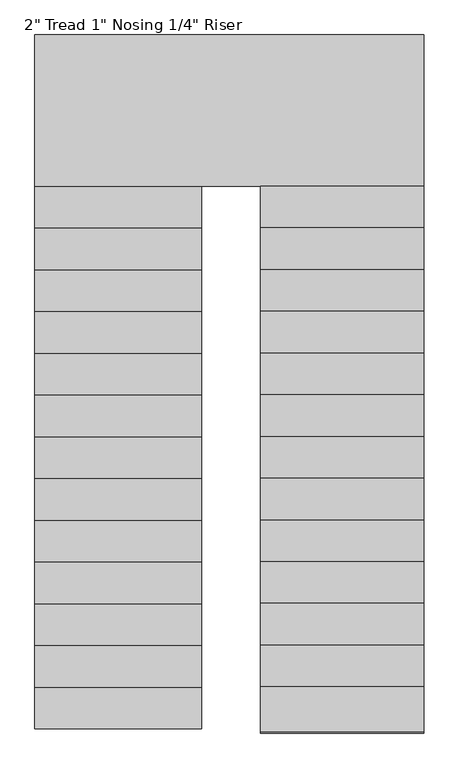
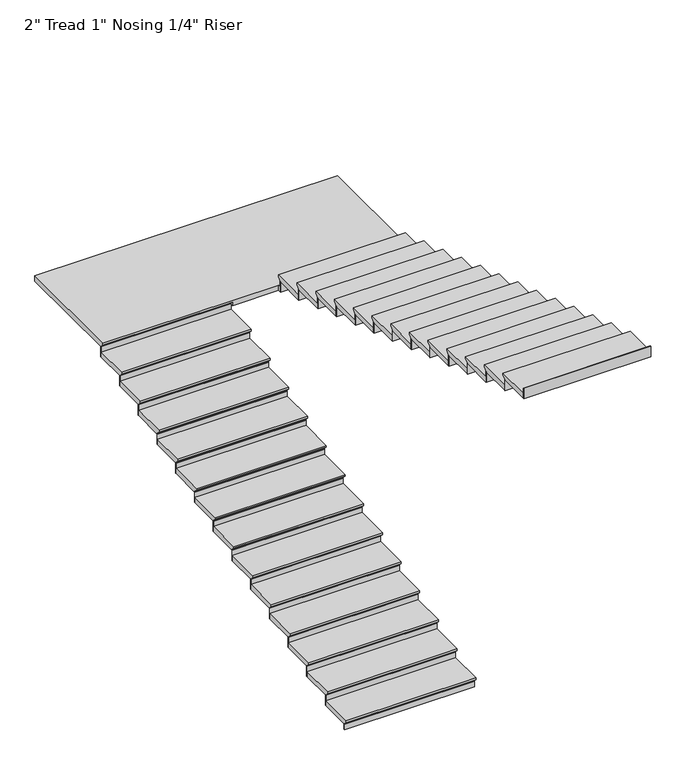
"""IFC4 building model written with IfcOpenShell, lengths in millimetres: stair flight geometry."""

from ifc_helpers import new_model, si_unit, origin, place, context, project, spatial, faceted_brep, source, transform, mapped, element, save


def stair_flight_1eae5bb9(model_context):
    return source(origin(), model_context, "Body", "Brep", [
        faceted_brep([(-629.5987998, 2564.5067329, 84.3642857), (-629.5987998, 2564.5067329, 103.4142857), (-1848.7987998, 2564.5067329, 103.4142857), (-1848.7987998, 2564.5067329, 84.3642857), (-629.5987998, 2589.9067329, 58.9642857), (-1848.7987998, 2589.9067329, 58.9642857), (-629.5987998, 2894.7067329, 103.4142857), (-1848.7987998, 2894.7067329, 103.4142857), (-1848.7987998, 2589.9067329, 52.6142857), (-1848.7987998, 2894.7067329, 52.6142857), (-629.5987998, 2894.7067329, 52.6142857), (-629.5987998, 2589.9067329, 52.6142857)], [[[0, 1, 2, 3]], [[4, 0, 3, 5]], [[2, 1, 6, 7]], [[8, 9, 10, 11]], [[2, 7, 9, 8, 5, 3]], [[8, 11, 4, 5]], [[6, 1, 0, 4, 11, 10]], [[7, 6, 10, 9]]]),
        faceted_brep([(-629.5987998, 2589.9067329, 52.6142857), (-629.5987998, 2589.9067329, 0.0), (-629.5987998, 2596.2567329, 0.0), (-629.5987998, 2596.2567329, 52.6142857), (-1848.7987998, 2589.9067329, 52.6142857), (-1848.7987998, 2596.2567329, 52.6142857), (-1848.7987998, 2596.2567329, 0.0), (-1848.7987998, 2589.9067329, 0.0)], [[[0, 1, 2, 3]], [[4, 5, 6, 7]], [[1, 0, 4, 7]], [[2, 1, 7, 6]], [[3, 2, 6, 5]], [[0, 3, 5, 4]]]),
        faceted_brep([(-629.5987998, 2894.7067329, 156.0285714), (-629.5987998, 2894.7067329, 52.6142857), (-629.5987998, 2901.0567329, 52.6142857), (-629.5987998, 2901.0567329, 156.0285714), (-1848.7987998, 2894.7067329, 156.0285714), (-1848.7987998, 2901.0567329, 156.0285714), (-1848.7987998, 2901.0567329, 52.6142857), (-1848.7987998, 2894.7067329, 52.6142857)], [[[0, 1, 2, 3]], [[4, 5, 6, 7]], [[1, 0, 4, 7]], [[2, 1, 7, 6]], [[3, 2, 6, 5]], [[0, 3, 5, 4]]]),
        faceted_brep([(-1848.7987998, 2869.3067329, 206.8285714), (-629.5987998, 2869.3067329, 206.8285714), (-629.5987998, 3199.5067329, 206.8285714), (-1848.7987998, 3199.5067329, 206.8285714), (-1848.7987998, 2894.7067329, 156.0285714), (-1848.7987998, 3199.5067329, 156.0285714), (-629.5987998, 3199.5067329, 156.0285714), (-629.5987998, 2894.7067329, 156.0285714), (-1848.7987998, 2894.7067329, 162.3785714), (-1848.7987998, 2869.3067329, 187.7785714), (-629.5987998, 2894.7067329, 162.3785714), (-629.5987998, 2869.3067329, 187.7785714)], [[[0, 1, 2, 3]], [[4, 5, 6, 7]], [[0, 3, 5, 4, 8, 9]], [[4, 7, 10, 8]], [[2, 1, 11, 10, 7, 6]], [[3, 2, 6, 5]], [[11, 1, 0, 9]], [[10, 11, 9, 8]]]),
        faceted_brep([(-629.5987998, 3199.5067329, 259.4428571), (-629.5987998, 3199.5067329, 156.0285714), (-629.5987998, 3205.8567329, 156.0285714), (-629.5987998, 3205.8567329, 259.4428571), (-1848.7987998, 3199.5067329, 259.4428571), (-1848.7987998, 3205.8567329, 259.4428571), (-1848.7987998, 3205.8567329, 156.0285714), (-1848.7987998, 3199.5067329, 156.0285714)], [[[0, 1, 2, 3]], [[4, 5, 6, 7]], [[1, 0, 4, 7]], [[2, 1, 7, 6]], [[3, 2, 6, 5]], [[0, 3, 5, 4]]]),
        faceted_brep([(-1848.7987998, 3174.1067329, 310.2428571), (-629.5987998, 3174.1067329, 310.2428571), (-629.5987998, 3504.3067329, 310.2428571), (-1848.7987998, 3504.3067329, 310.2428571), (-1848.7987998, 3199.5067329, 259.4428571), (-1848.7987998, 3504.3067329, 259.4428571), (-629.5987998, 3504.3067329, 259.4428571), (-629.5987998, 3199.5067329, 259.4428571), (-1848.7987998, 3199.5067329, 265.7928571), (-1848.7987998, 3174.1067329, 291.1928571), (-629.5987998, 3199.5067329, 265.7928571), (-629.5987998, 3174.1067329, 291.1928571)], [[[0, 1, 2, 3]], [[4, 5, 6, 7]], [[0, 3, 5, 4, 8, 9]], [[4, 7, 10, 8]], [[2, 1, 11, 10, 7, 6]], [[3, 2, 6, 5]], [[11, 1, 0, 9]], [[10, 11, 9, 8]]]),
        faceted_brep([(-629.5987998, 3504.3067329, 362.8571429), (-629.5987998, 3504.3067329, 259.4428571), (-629.5987998, 3510.6567329, 259.4428571), (-629.5987998, 3510.6567329, 362.8571429), (-1848.7987998, 3504.3067329, 362.8571429), (-1848.7987998, 3510.6567329, 362.8571429), (-1848.7987998, 3510.6567329, 259.4428571), (-1848.7987998, 3504.3067329, 259.4428571)], [[[0, 1, 2, 3]], [[4, 5, 6, 7]], [[1, 0, 4, 7]], [[2, 1, 7, 6]], [[3, 2, 6, 5]], [[0, 3, 5, 4]]]),
        faceted_brep([(-1848.7987998, 3478.9067329, 413.6571429), (-629.5987998, 3478.9067329, 413.6571429), (-629.5987998, 3809.1067329, 413.6571429), (-1848.7987998, 3809.1067329, 413.6571429), (-1848.7987998, 3504.3067329, 362.8571429), (-1848.7987998, 3809.1067329, 362.8571429), (-629.5987998, 3809.1067329, 362.8571429), (-629.5987998, 3504.3067329, 362.8571429), (-1848.7987998, 3504.3067329, 369.2071429), (-1848.7987998, 3478.9067329, 394.6071429), (-629.5987998, 3504.3067329, 369.2071429), (-629.5987998, 3478.9067329, 394.6071429)], [[[0, 1, 2, 3]], [[4, 5, 6, 7]], [[0, 3, 5, 4, 8, 9]], [[4, 7, 10, 8]], [[2, 1, 11, 10, 7, 6]], [[3, 2, 6, 5]], [[11, 1, 0, 9]], [[10, 11, 9, 8]]]),
        faceted_brep([(-629.5987998, 3809.1067329, 466.2714286), (-629.5987998, 3809.1067329, 362.8571429), (-629.5987998, 3815.4567329, 362.8571429), (-629.5987998, 3815.4567329, 466.2714286), (-1848.7987998, 3809.1067329, 466.2714286), (-1848.7987998, 3815.4567329, 466.2714286), (-1848.7987998, 3815.4567329, 362.8571429), (-1848.7987998, 3809.1067329, 362.8571429)], [[[0, 1, 2, 3]], [[4, 5, 6, 7]], [[1, 0, 4, 7]], [[2, 1, 7, 6]], [[3, 2, 6, 5]], [[0, 3, 5, 4]]]),
        faceted_brep([(-1848.7987998, 3783.7067329, 517.0714286), (-629.5987998, 3783.7067329, 517.0714286), (-629.5987998, 4113.9067329, 517.0714286), (-1848.7987998, 4113.9067329, 517.0714286), (-1848.7987998, 3809.1067329, 466.2714286), (-1848.7987998, 4113.9067329, 466.2714286), (-629.5987998, 4113.9067329, 466.2714286), (-629.5987998, 3809.1067329, 466.2714286), (-1848.7987998, 3809.1067329, 472.6214286), (-1848.7987998, 3783.7067329, 498.0214286), (-629.5987998, 3809.1067329, 472.6214286), (-629.5987998, 3783.7067329, 498.0214286)], [[[0, 1, 2, 3]], [[4, 5, 6, 7]], [[0, 3, 5, 4, 8, 9]], [[4, 7, 10, 8]], [[2, 1, 11, 10, 7, 6]], [[3, 2, 6, 5]], [[11, 1, 0, 9]], [[10, 11, 9, 8]]]),
        faceted_brep([(-629.5987998, 4113.9067329, 569.6857143), (-629.5987998, 4113.9067329, 466.2714286), (-629.5987998, 4120.2567329, 466.2714286), (-629.5987998, 4120.2567329, 569.6857143), (-1848.7987998, 4113.9067329, 569.6857143), (-1848.7987998, 4120.2567329, 569.6857143), (-1848.7987998, 4120.2567329, 466.2714286), (-1848.7987998, 4113.9067329, 466.2714286)], [[[0, 1, 2, 3]], [[4, 5, 6, 7]], [[1, 0, 4, 7]], [[2, 1, 7, 6]], [[3, 2, 6, 5]], [[0, 3, 5, 4]]]),
        faceted_brep([(-1848.7987998, 4088.5067329, 620.4857143), (-629.5987998, 4088.5067329, 620.4857143), (-629.5987998, 4418.7067329, 620.4857143), (-1848.7987998, 4418.7067329, 620.4857143), (-1848.7987998, 4113.9067329, 569.6857143), (-1848.7987998, 4418.7067329, 569.6857143), (-629.5987998, 4418.7067329, 569.6857143), (-629.5987998, 4113.9067329, 569.6857143), (-1848.7987998, 4113.9067329, 576.0357143), (-1848.7987998, 4088.5067329, 601.4357143), (-629.5987998, 4113.9067329, 576.0357143), (-629.5987998, 4088.5067329, 601.4357143)], [[[0, 1, 2, 3]], [[4, 5, 6, 7]], [[0, 3, 5, 4, 8, 9]], [[4, 7, 10, 8]], [[2, 1, 11, 10, 7, 6]], [[3, 2, 6, 5]], [[11, 1, 0, 9]], [[10, 11, 9, 8]]]),
        faceted_brep([(-629.5987998, 4418.7067329, 673.1), (-629.5987998, 4418.7067329, 569.6857143), (-629.5987998, 4425.0567329, 569.6857143), (-629.5987998, 4425.0567329, 673.1), (-1848.7987998, 4418.7067329, 673.1), (-1848.7987998, 4425.0567329, 673.1), (-1848.7987998, 4425.0567329, 569.6857143), (-1848.7987998, 4418.7067329, 569.6857143)], [[[0, 1, 2, 3]], [[4, 5, 6, 7]], [[1, 0, 4, 7]], [[2, 1, 7, 6]], [[3, 2, 6, 5]], [[0, 3, 5, 4]]]),
        faceted_brep([(-1848.7987998, 4393.3067329, 723.9), (-629.5987998, 4393.3067329, 723.9), (-629.5987998, 4723.5067329, 723.9), (-1848.7987998, 4723.5067329, 723.9), (-1848.7987998, 4418.7067329, 673.1), (-1848.7987998, 4723.5067329, 673.1), (-629.5987998, 4723.5067329, 673.1), (-629.5987998, 4418.7067329, 673.1), (-1848.7987998, 4418.7067329, 679.45), (-1848.7987998, 4393.3067329, 704.85), (-629.5987998, 4418.7067329, 679.45), (-629.5987998, 4393.3067329, 704.85)], [[[0, 1, 2, 3]], [[4, 5, 6, 7]], [[0, 3, 5, 4, 8, 9]], [[4, 7, 10, 8]], [[2, 1, 11, 10, 7, 6]], [[3, 2, 6, 5]], [[11, 1, 0, 9]], [[10, 11, 9, 8]]]),
        faceted_brep([(-629.5987998, 4723.5067329, 776.5142857), (-629.5987998, 4723.5067329, 673.1), (-629.5987998, 4729.8567329, 673.1), (-629.5987998, 4729.8567329, 776.5142857), (-1848.7987998, 4723.5067329, 776.5142857), (-1848.7987998, 4729.8567329, 776.5142857), (-1848.7987998, 4729.8567329, 673.1), (-1848.7987998, 4723.5067329, 673.1)], [[[0, 1, 2, 3]], [[4, 5, 6, 7]], [[1, 0, 4, 7]], [[2, 1, 7, 6]], [[3, 2, 6, 5]], [[0, 3, 5, 4]]]),
        faceted_brep([(-1848.7987998, 4698.1067329, 827.3142857), (-629.5987998, 4698.1067329, 827.3142857), (-629.5987998, 5028.3067329, 827.3142857), (-1848.7987998, 5028.3067329, 827.3142857), (-1848.7987998, 4723.5067329, 776.5142857), (-1848.7987998, 5028.3067329, 776.5142857), (-629.5987998, 5028.3067329, 776.5142857), (-629.5987998, 4723.5067329, 776.5142857), (-1848.7987998, 4723.5067329, 782.8642857), (-1848.7987998, 4698.1067329, 808.2642857), (-629.5987998, 4723.5067329, 782.8642857), (-629.5987998, 4698.1067329, 808.2642857)], [[[0, 1, 2, 3]], [[4, 5, 6, 7]], [[0, 3, 5, 4, 8, 9]], [[4, 7, 10, 8]], [[2, 1, 11, 10, 7, 6]], [[3, 2, 6, 5]], [[11, 1, 0, 9]], [[10, 11, 9, 8]]]),
        faceted_brep([(-629.5987998, 5028.3067329, 879.9285714), (-629.5987998, 5028.3067329, 776.5142857), (-629.5987998, 5034.6567329, 776.5142857), (-629.5987998, 5034.6567329, 879.9285714), (-1848.7987998, 5028.3067329, 879.9285714), (-1848.7987998, 5034.6567329, 879.9285714), (-1848.7987998, 5034.6567329, 776.5142857), (-1848.7987998, 5028.3067329, 776.5142857)], [[[0, 1, 2, 3]], [[4, 5, 6, 7]], [[1, 0, 4, 7]], [[2, 1, 7, 6]], [[3, 2, 6, 5]], [[0, 3, 5, 4]]]),
        faceted_brep([(-1848.7987998, 5002.9067329, 930.7285714), (-629.5987998, 5002.9067329, 930.7285714), (-629.5987998, 5333.1067329, 930.7285714), (-1848.7987998, 5333.1067329, 930.7285714), (-1848.7987998, 5028.3067329, 879.9285714), (-1848.7987998, 5333.1067329, 879.9285714), (-629.5987998, 5333.1067329, 879.9285714), (-629.5987998, 5028.3067329, 879.9285714), (-1848.7987998, 5028.3067329, 886.2785714), (-1848.7987998, 5002.9067329, 911.6785714), (-629.5987998, 5028.3067329, 886.2785714), (-629.5987998, 5002.9067329, 911.6785714)], [[[0, 1, 2, 3]], [[4, 5, 6, 7]], [[0, 3, 5, 4, 8, 9]], [[4, 7, 10, 8]], [[2, 1, 11, 10, 7, 6]], [[3, 2, 6, 5]], [[11, 1, 0, 9]], [[10, 11, 9, 8]]]),
        faceted_brep([(-629.5987998, 5333.1067329, 983.3428571), (-629.5987998, 5333.1067329, 879.9285714), (-629.5987998, 5339.4567329, 879.9285714), (-629.5987998, 5339.4567329, 983.3428571), (-1848.7987998, 5333.1067329, 983.3428571), (-1848.7987998, 5339.4567329, 983.3428571), (-1848.7987998, 5339.4567329, 879.9285714), (-1848.7987998, 5333.1067329, 879.9285714)], [[[0, 1, 2, 3]], [[4, 5, 6, 7]], [[1, 0, 4, 7]], [[2, 1, 7, 6]], [[3, 2, 6, 5]], [[0, 3, 5, 4]]]),
        faceted_brep([(-1848.7987998, 5307.7067329, 1034.1428571), (-629.5987998, 5307.7067329, 1034.1428571), (-629.5987998, 5637.9067329, 1034.1428571), (-1848.7987998, 5637.9067329, 1034.1428571), (-1848.7987998, 5333.1067329, 983.3428571), (-1848.7987998, 5637.9067329, 983.3428571), (-629.5987998, 5637.9067329, 983.3428571), (-629.5987998, 5333.1067329, 983.3428571), (-1848.7987998, 5333.1067329, 989.6928571), (-1848.7987998, 5307.7067329, 1015.0928571), (-629.5987998, 5333.1067329, 989.6928571), (-629.5987998, 5307.7067329, 1015.0928571)], [[[0, 1, 2, 3]], [[4, 5, 6, 7]], [[0, 3, 5, 4, 8, 9]], [[4, 7, 10, 8]], [[2, 1, 11, 10, 7, 6]], [[3, 2, 6, 5]], [[11, 1, 0, 9]], [[10, 11, 9, 8]]]),
        faceted_brep([(-629.5987998, 5637.9067329, 1086.7571429), (-629.5987998, 5637.9067329, 983.3428571), (-629.5987998, 5644.2567329, 983.3428571), (-629.5987998, 5644.2567329, 1086.7571429), (-1848.7987998, 5637.9067329, 1086.7571429), (-1848.7987998, 5644.2567329, 1086.7571429), (-1848.7987998, 5644.2567329, 983.3428571), (-1848.7987998, 5637.9067329, 983.3428571)], [[[0, 1, 2, 3]], [[4, 5, 6, 7]], [[1, 0, 4, 7]], [[2, 1, 7, 6]], [[3, 2, 6, 5]], [[0, 3, 5, 4]]]),
        faceted_brep([(-1848.7987998, 5612.5067329, 1137.5571429), (-629.5987998, 5612.5067329, 1137.5571429), (-629.5987998, 5942.7067329, 1137.5571429), (-1848.7987998, 5942.7067329, 1137.5571429), (-1848.7987998, 5637.9067329, 1086.7571429), (-1848.7987998, 5942.7067329, 1086.7571429), (-629.5987998, 5942.7067329, 1086.7571429), (-629.5987998, 5637.9067329, 1086.7571429), (-1848.7987998, 5637.9067329, 1093.1071429), (-1848.7987998, 5612.5067329, 1118.5071429), (-629.5987998, 5637.9067329, 1093.1071429), (-629.5987998, 5612.5067329, 1118.5071429)], [[[0, 1, 2, 3]], [[4, 5, 6, 7]], [[0, 3, 5, 4, 8, 9]], [[4, 7, 10, 8]], [[2, 1, 11, 10, 7, 6]], [[3, 2, 6, 5]], [[11, 1, 0, 9]], [[10, 11, 9, 8]]]),
        faceted_brep([(-629.5987998, 5942.7067329, 1190.1714286), (-629.5987998, 5942.7067329, 1086.7571429), (-629.5987998, 5949.0567329, 1086.7571429), (-629.5987998, 5949.0567329, 1190.1714286), (-1848.7987998, 5942.7067329, 1190.1714286), (-1848.7987998, 5949.0567329, 1190.1714286), (-1848.7987998, 5949.0567329, 1086.7571429), (-1848.7987998, 5942.7067329, 1086.7571429)], [[[0, 1, 2, 3]], [[4, 5, 6, 7]], [[1, 0, 4, 7]], [[2, 1, 7, 6]], [[3, 2, 6, 5]], [[0, 3, 5, 4]]]),
        faceted_brep([(-1848.7987998, 5917.3067329, 1240.9714286), (-629.5987998, 5917.3067329, 1240.9714286), (-629.5987998, 6247.5067329, 1240.9714286), (-1848.7987998, 6247.5067329, 1240.9714286), (-1848.7987998, 5942.7067329, 1190.1714286), (-1848.7987998, 6247.5067329, 1190.1714286), (-629.5987998, 6247.5067329, 1190.1714286), (-629.5987998, 5942.7067329, 1190.1714286), (-1848.7987998, 5942.7067329, 1196.5214286), (-1848.7987998, 5917.3067329, 1221.9214286), (-629.5987998, 5942.7067329, 1196.5214286), (-629.5987998, 5917.3067329, 1221.9214286)], [[[0, 1, 2, 3]], [[4, 5, 6, 7]], [[0, 3, 5, 4, 8, 9]], [[4, 7, 10, 8]], [[2, 1, 11, 10, 7, 6]], [[3, 2, 6, 5]], [[11, 1, 0, 9]], [[10, 11, 9, 8]]]),
        faceted_brep([(-629.5987998, 6247.5067329, 1293.5857143), (-629.5987998, 6247.5067329, 1190.1714286), (-629.5987998, 6253.8567329, 1190.1714286), (-629.5987998, 6253.8567329, 1293.5857143), (-1848.7987998, 6247.5067329, 1293.5857143), (-1848.7987998, 6253.8567329, 1293.5857143), (-1848.7987998, 6253.8567329, 1190.1714286), (-1848.7987998, 6247.5067329, 1190.1714286)], [[[0, 1, 2, 3]], [[4, 5, 6, 7]], [[1, 0, 4, 7]], [[2, 1, 7, 6]], [[3, 2, 6, 5]], [[0, 3, 5, 4]]]),
        faceted_brep([(-1848.7987998, 6222.1067329, 1344.3857143), (-629.5987998, 6222.1067329, 1344.3857143), (-629.5987998, 6552.3067329, 1344.3857143), (-1848.7987998, 6552.3067329, 1344.3857143), (-1848.7987998, 6247.5067329, 1293.5857143), (-1848.7987998, 6552.3067329, 1293.5857143), (-629.5987998, 6552.3067329, 1293.5857143), (-629.5987998, 6247.5067329, 1293.5857143), (-1848.7987998, 6247.5067329, 1299.9357143), (-1848.7987998, 6222.1067329, 1325.3357143), (-629.5987998, 6247.5067329, 1299.9357143), (-629.5987998, 6222.1067329, 1325.3357143)], [[[0, 1, 2, 3]], [[4, 5, 6, 7]], [[0, 3, 5, 4, 8, 9]], [[4, 7, 10, 8]], [[2, 1, 11, 10, 7, 6]], [[3, 2, 6, 5]], [[11, 1, 0, 9]], [[10, 11, 9, 8]]]),
        faceted_brep([(-629.5987998, 6552.3067329, 1397.0), (-629.5987998, 6552.3067329, 1293.5857143), (-629.5987998, 6558.6567329, 1293.5857143), (-629.5987998, 6558.6567329, 1397.0), (-1848.7987998, 6552.3067329, 1397.0), (-1848.7987998, 6558.6567329, 1397.0), (-1848.7987998, 6558.6567329, 1293.5857143), (-1848.7987998, 6552.3067329, 1293.5857143)], [[[0, 1, 2, 3]], [[4, 5, 6, 7]], [[1, 0, 4, 7]], [[2, 1, 7, 6]], [[3, 2, 6, 5]], [[0, 3, 5, 4]]]),
        faceted_brep([(996.0012002, 6501.5067329, 1447.8), (996.0012002, 7631.8067329, 1447.8), (-1848.7987998, 7631.8067329, 1447.8), (-1848.7987998, 6526.9067329, 1447.8), (-197.7987915, 6526.9067329, 1447.8), (-197.7987915, 6501.5067329, 1447.8), (996.0012002, 7631.8067329, 1397.0), (996.0012002, 6501.5067329, 1397.0), (-197.7987915, 6501.5067329, 1397.0), (-197.7987915, 6526.9067329, 1397.0), (-629.5987998, 6526.9067329, 1397.0), (-629.5987998, 6552.3067329, 1397.0), (-1848.7987998, 6552.3067329, 1397.0), (-1848.7987998, 7631.8067329, 1397.0), (-629.5987998, 6552.3067329, 1403.35), (-1848.7987998, 6552.3067329, 1403.35), (-1848.7987998, 6526.9067329, 1428.75), (-629.5987998, 6526.9067329, 1428.75)], [[[0, 1, 2, 3, 4, 5]], [[6, 7, 8, 9, 10, 11, 12, 13]], [[1, 0, 7, 6]], [[2, 1, 6, 13]], [[12, 11, 14, 15]], [[4, 3, 16, 17, 10, 9]], [[5, 4, 9, 8]], [[0, 5, 8, 7]], [[16, 15, 14, 17]], [[3, 2, 13, 12, 15, 16]], [[11, 10, 17, 14]]]),
        faceted_brep([(-197.7987915, 6501.5067329, 1500.4142857), (-197.7987915, 6501.5067329, 1397.0), (-197.7987915, 6495.1567329, 1397.0), (-197.7987915, 6495.1567329, 1500.4142857), (996.0012002, 6501.5067329, 1500.4142857), (996.0012002, 6495.1567329, 1500.4142857), (996.0012002, 6495.1567329, 1397.0), (996.0012002, 6501.5067329, 1397.0)], [[[0, 1, 2, 3]], [[4, 5, 6, 7]], [[1, 0, 4, 7]], [[2, 1, 7, 6]], [[3, 2, 6, 5]], [[0, 3, 5, 4]]]),
        faceted_brep([(996.0012002, 6526.9067329, 1551.2142857), (-197.7987915, 6526.9067329, 1551.2142857), (-197.7987915, 6196.7067329, 1551.2142857), (996.0012002, 6196.7067329, 1551.2142857), (996.0012002, 6501.5067329, 1500.4142857), (996.0012002, 6196.7067329, 1500.4142857), (-197.7987915, 6196.7067329, 1500.4142857), (-197.7987915, 6501.5067329, 1500.4142857), (996.0012002, 6501.5067329, 1506.7642857), (996.0012002, 6526.9067329, 1532.1642857), (-197.7987915, 6501.5067329, 1506.7642857), (-197.7987915, 6526.9067329, 1532.1642857)], [[[0, 1, 2, 3]], [[4, 5, 6, 7]], [[0, 3, 5, 4, 8, 9]], [[4, 7, 10, 8]], [[2, 1, 11, 10, 7, 6]], [[3, 2, 6, 5]], [[11, 1, 0, 9]], [[10, 11, 9, 8]]]),
        faceted_brep([(-197.7987915, 6196.7067329, 1603.8285714), (-197.7987915, 6196.7067329, 1500.4142857), (-197.7987915, 6190.3567329, 1500.4142857), (-197.7987915, 6190.3567329, 1603.8285714), (996.0012002, 6196.7067329, 1603.8285714), (996.0012002, 6190.3567329, 1603.8285714), (996.0012002, 6190.3567329, 1500.4142857), (996.0012002, 6196.7067329, 1500.4142857)], [[[0, 1, 2, 3]], [[4, 5, 6, 7]], [[1, 0, 4, 7]], [[2, 1, 7, 6]], [[3, 2, 6, 5]], [[0, 3, 5, 4]]]),
        faceted_brep([(996.0012002, 6222.1067329, 1654.6285714), (-197.7987915, 6222.1067329, 1654.6285714), (-197.7987915, 5891.9067329, 1654.6285714), (996.0012002, 5891.9067329, 1654.6285714), (996.0012002, 6196.7067329, 1603.8285714), (996.0012002, 5891.9067329, 1603.8285714), (-197.7987915, 5891.9067329, 1603.8285714), (-197.7987915, 6196.7067329, 1603.8285714), (996.0012002, 6196.7067329, 1610.1785714), (996.0012002, 6222.1067329, 1635.5785714), (-197.7987915, 6196.7067329, 1610.1785714), (-197.7987915, 6222.1067329, 1635.5785714)], [[[0, 1, 2, 3]], [[4, 5, 6, 7]], [[0, 3, 5, 4, 8, 9]], [[4, 7, 10, 8]], [[2, 1, 11, 10, 7, 6]], [[3, 2, 6, 5]], [[11, 1, 0, 9]], [[10, 11, 9, 8]]]),
        faceted_brep([(-197.7987915, 5891.9067329, 1707.2428571), (-197.7987915, 5891.9067329, 1603.8285714), (-197.7987915, 5885.5567329, 1603.8285714), (-197.7987915, 5885.5567329, 1707.2428571), (996.0012002, 5891.9067329, 1707.2428571), (996.0012002, 5885.5567329, 1707.2428571), (996.0012002, 5885.5567329, 1603.8285714), (996.0012002, 5891.9067329, 1603.8285714)], [[[0, 1, 2, 3]], [[4, 5, 6, 7]], [[1, 0, 4, 7]], [[2, 1, 7, 6]], [[3, 2, 6, 5]], [[0, 3, 5, 4]]]),
        faceted_brep([(996.0012002, 5917.3067329, 1758.0428571), (-197.7987915, 5917.3067329, 1758.0428571), (-197.7987915, 5587.1067329, 1758.0428571), (996.0012002, 5587.1067329, 1758.0428571), (996.0012002, 5891.9067329, 1707.2428571), (996.0012002, 5587.1067329, 1707.2428571), (-197.7987915, 5587.1067329, 1707.2428571), (-197.7987915, 5891.9067329, 1707.2428571), (996.0012002, 5891.9067329, 1713.5928571), (996.0012002, 5917.3067329, 1738.9928571), (-197.7987915, 5891.9067329, 1713.5928571), (-197.7987915, 5917.3067329, 1738.9928571)], [[[0, 1, 2, 3]], [[4, 5, 6, 7]], [[0, 3, 5, 4, 8, 9]], [[4, 7, 10, 8]], [[2, 1, 11, 10, 7, 6]], [[3, 2, 6, 5]], [[11, 1, 0, 9]], [[10, 11, 9, 8]]]),
        faceted_brep([(-197.7987915, 5587.1067329, 1810.6571429), (-197.7987915, 5587.1067329, 1707.2428571), (-197.7987915, 5580.7567329, 1707.2428571), (-197.7987915, 5580.7567329, 1810.6571429), (996.0012002, 5587.1067329, 1810.6571429), (996.0012002, 5580.7567329, 1810.6571429), (996.0012002, 5580.7567329, 1707.2428571), (996.0012002, 5587.1067329, 1707.2428571)], [[[0, 1, 2, 3]], [[4, 5, 6, 7]], [[1, 0, 4, 7]], [[2, 1, 7, 6]], [[3, 2, 6, 5]], [[0, 3, 5, 4]]]),
        faceted_brep([(996.0012002, 5612.5067329, 1861.4571429), (-197.7987915, 5612.5067329, 1861.4571429), (-197.7987915, 5282.3067329, 1861.4571429), (996.0012002, 5282.3067329, 1861.4571429), (996.0012002, 5587.1067329, 1810.6571429), (996.0012002, 5282.3067329, 1810.6571429), (-197.7987915, 5282.3067329, 1810.6571429), (-197.7987915, 5587.1067329, 1810.6571429), (996.0012002, 5587.1067329, 1817.0071429), (996.0012002, 5612.5067329, 1842.4071429), (-197.7987915, 5587.1067329, 1817.0071429), (-197.7987915, 5612.5067329, 1842.4071429)], [[[0, 1, 2, 3]], [[4, 5, 6, 7]], [[0, 3, 5, 4, 8, 9]], [[4, 7, 10, 8]], [[2, 1, 11, 10, 7, 6]], [[3, 2, 6, 5]], [[11, 1, 0, 9]], [[10, 11, 9, 8]]]),
        faceted_brep([(-197.7987915, 5282.3067329, 1914.0714286), (-197.7987915, 5282.3067329, 1810.6571429), (-197.7987915, 5275.9567329, 1810.6571429), (-197.7987915, 5275.9567329, 1914.0714286), (996.0012002, 5282.3067329, 1914.0714286), (996.0012002, 5275.9567329, 1914.0714286), (996.0012002, 5275.9567329, 1810.6571429), (996.0012002, 5282.3067329, 1810.6571429)], [[[0, 1, 2, 3]], [[4, 5, 6, 7]], [[1, 0, 4, 7]], [[2, 1, 7, 6]], [[3, 2, 6, 5]], [[0, 3, 5, 4]]]),
        faceted_brep([(996.0012002, 5307.7067329, 1964.8714286), (-197.7987915, 5307.7067329, 1964.8714286), (-197.7987915, 4977.5067329, 1964.8714286), (996.0012002, 4977.5067329, 1964.8714286), (996.0012002, 5282.3067329, 1914.0714286), (996.0012002, 4977.5067329, 1914.0714286), (-197.7987915, 4977.5067329, 1914.0714286), (-197.7987915, 5282.3067329, 1914.0714286), (996.0012002, 5282.3067329, 1920.4214286), (996.0012002, 5307.7067329, 1945.8214286), (-197.7987915, 5282.3067329, 1920.4214286), (-197.7987915, 5307.7067329, 1945.8214286)], [[[0, 1, 2, 3]], [[4, 5, 6, 7]], [[0, 3, 5, 4, 8, 9]], [[4, 7, 10, 8]], [[2, 1, 11, 10, 7, 6]], [[3, 2, 6, 5]], [[11, 1, 0, 9]], [[10, 11, 9, 8]]]),
        faceted_brep([(-197.7987915, 4977.5067329, 2017.4857143), (-197.7987915, 4977.5067329, 1914.0714286), (-197.7987915, 4971.1567329, 1914.0714286), (-197.7987915, 4971.1567329, 2017.4857143), (996.0012002, 4977.5067329, 2017.4857143), (996.0012002, 4971.1567329, 2017.4857143), (996.0012002, 4971.1567329, 1914.0714286), (996.0012002, 4977.5067329, 1914.0714286)], [[[0, 1, 2, 3]], [[4, 5, 6, 7]], [[1, 0, 4, 7]], [[2, 1, 7, 6]], [[3, 2, 6, 5]], [[0, 3, 5, 4]]]),
        faceted_brep([(996.0012002, 5002.9067329, 2068.2857143), (-197.7987915, 5002.9067329, 2068.2857143), (-197.7987915, 4672.7067329, 2068.2857143), (996.0012002, 4672.7067329, 2068.2857143), (996.0012002, 4977.5067329, 2017.4857143), (996.0012002, 4672.7067329, 2017.4857143), (-197.7987915, 4672.7067329, 2017.4857143), (-197.7987915, 4977.5067329, 2017.4857143), (996.0012002, 4977.5067329, 2023.8357143), (996.0012002, 5002.9067329, 2049.2357143), (-197.7987915, 4977.5067329, 2023.8357143), (-197.7987915, 5002.9067329, 2049.2357143)], [[[0, 1, 2, 3]], [[4, 5, 6, 7]], [[0, 3, 5, 4, 8, 9]], [[4, 7, 10, 8]], [[2, 1, 11, 10, 7, 6]], [[3, 2, 6, 5]], [[11, 1, 0, 9]], [[10, 11, 9, 8]]]),
        faceted_brep([(-197.7987915, 4672.7067329, 2120.9), (-197.7987915, 4672.7067329, 2017.4857143), (-197.7987915, 4666.3567329, 2017.4857143), (-197.7987915, 4666.3567329, 2120.9), (996.0012002, 4672.7067329, 2120.9), (996.0012002, 4666.3567329, 2120.9), (996.0012002, 4666.3567329, 2017.4857143), (996.0012002, 4672.7067329, 2017.4857143)], [[[0, 1, 2, 3]], [[4, 5, 6, 7]], [[1, 0, 4, 7]], [[2, 1, 7, 6]], [[3, 2, 6, 5]], [[0, 3, 5, 4]]]),
        faceted_brep([(996.0012002, 4698.1067329, 2171.7), (-197.7987915, 4698.1067329, 2171.7), (-197.7987915, 4367.9067329, 2171.7), (996.0012002, 4367.9067329, 2171.7), (996.0012002, 4672.7067329, 2120.9), (996.0012002, 4367.9067329, 2120.9), (-197.7987915, 4367.9067329, 2120.9), (-197.7987915, 4672.7067329, 2120.9), (996.0012002, 4672.7067329, 2127.25), (996.0012002, 4698.1067329, 2152.65), (-197.7987915, 4672.7067329, 2127.25), (-197.7987915, 4698.1067329, 2152.65)], [[[0, 1, 2, 3]], [[4, 5, 6, 7]], [[0, 3, 5, 4, 8, 9]], [[4, 7, 10, 8]], [[2, 1, 11, 10, 7, 6]], [[3, 2, 6, 5]], [[11, 1, 0, 9]], [[10, 11, 9, 8]]]),
        faceted_brep([(-197.7987915, 4367.9067329, 2224.3142857), (-197.7987915, 4367.9067329, 2120.9), (-197.7987915, 4361.5567329, 2120.9), (-197.7987915, 4361.5567329, 2224.3142857), (996.0012002, 4367.9067329, 2224.3142857), (996.0012002, 4361.5567329, 2224.3142857), (996.0012002, 4361.5567329, 2120.9), (996.0012002, 4367.9067329, 2120.9)], [[[0, 1, 2, 3]], [[4, 5, 6, 7]], [[1, 0, 4, 7]], [[2, 1, 7, 6]], [[3, 2, 6, 5]], [[0, 3, 5, 4]]]),
        faceted_brep([(996.0012002, 4393.3067329, 2275.1142857), (-197.7987915, 4393.3067329, 2275.1142857), (-197.7987915, 4063.1067329, 2275.1142857), (996.0012002, 4063.1067329, 2275.1142857), (996.0012002, 4367.9067329, 2224.3142857), (996.0012002, 4063.1067329, 2224.3142857), (-197.7987915, 4063.1067329, 2224.3142857), (-197.7987915, 4367.9067329, 2224.3142857), (996.0012002, 4367.9067329, 2230.6642857), (996.0012002, 4393.3067329, 2256.0642857), (-197.7987915, 4367.9067329, 2230.6642857), (-197.7987915, 4393.3067329, 2256.0642857)], [[[0, 1, 2, 3]], [[4, 5, 6, 7]], [[0, 3, 5, 4, 8, 9]], [[4, 7, 10, 8]], [[2, 1, 11, 10, 7, 6]], [[3, 2, 6, 5]], [[11, 1, 0, 9]], [[10, 11, 9, 8]]]),
        faceted_brep([(-197.7987915, 4063.1067329, 2327.7285714), (-197.7987915, 4063.1067329, 2224.3142857), (-197.7987915, 4056.7567329, 2224.3142857), (-197.7987915, 4056.7567329, 2327.7285714), (996.0012002, 4063.1067329, 2327.7285714), (996.0012002, 4056.7567329, 2327.7285714), (996.0012002, 4056.7567329, 2224.3142857), (996.0012002, 4063.1067329, 2224.3142857)], [[[0, 1, 2, 3]], [[4, 5, 6, 7]], [[1, 0, 4, 7]], [[2, 1, 7, 6]], [[3, 2, 6, 5]], [[0, 3, 5, 4]]]),
        faceted_brep([(996.0012002, 4088.5067329, 2378.5285714), (-197.7987915, 4088.5067329, 2378.5285714), (-197.7987915, 3758.3067329, 2378.5285714), (996.0012002, 3758.3067329, 2378.5285714), (996.0012002, 4063.1067329, 2327.7285714), (996.0012002, 3758.3067329, 2327.7285714), (-197.7987915, 3758.3067329, 2327.7285714), (-197.7987915, 4063.1067329, 2327.7285714), (996.0012002, 4063.1067329, 2334.0785714), (996.0012002, 4088.5067329, 2359.4785714), (-197.7987915, 4063.1067329, 2334.0785714), (-197.7987915, 4088.5067329, 2359.4785714)], [[[0, 1, 2, 3]], [[4, 5, 6, 7]], [[0, 3, 5, 4, 8, 9]], [[4, 7, 10, 8]], [[2, 1, 11, 10, 7, 6]], [[3, 2, 6, 5]], [[11, 1, 0, 9]], [[10, 11, 9, 8]]]),
        faceted_brep([(-197.7987915, 3758.3067329, 2431.1428571), (-197.7987915, 3758.3067329, 2327.7285714), (-197.7987915, 3751.9567329, 2327.7285714), (-197.7987915, 3751.9567329, 2431.1428571), (996.0012002, 3758.3067329, 2431.1428571), (996.0012002, 3751.9567329, 2431.1428571), (996.0012002, 3751.9567329, 2327.7285714), (996.0012002, 3758.3067329, 2327.7285714)], [[[0, 1, 2, 3]], [[4, 5, 6, 7]], [[1, 0, 4, 7]], [[2, 1, 7, 6]], [[3, 2, 6, 5]], [[0, 3, 5, 4]]]),
        faceted_brep([(996.0012002, 3783.7067329, 2481.9428571), (-197.7987915, 3783.7067329, 2481.9428571), (-197.7987915, 3453.5067329, 2481.9428571), (996.0012002, 3453.5067329, 2481.9428571), (996.0012002, 3758.3067329, 2431.1428571), (996.0012002, 3453.5067329, 2431.1428571), (-197.7987915, 3453.5067329, 2431.1428571), (-197.7987915, 3758.3067329, 2431.1428571), (996.0012002, 3758.3067329, 2437.4928571), (996.0012002, 3783.7067329, 2462.8928571), (-197.7987915, 3758.3067329, 2437.4928571), (-197.7987915, 3783.7067329, 2462.8928571)], [[[0, 1, 2, 3]], [[4, 5, 6, 7]], [[0, 3, 5, 4, 8, 9]], [[4, 7, 10, 8]], [[2, 1, 11, 10, 7, 6]], [[3, 2, 6, 5]], [[11, 1, 0, 9]], [[10, 11, 9, 8]]]),
        faceted_brep([(-197.7987915, 3453.5067329, 2534.5571429), (-197.7987915, 3453.5067329, 2431.1428571), (-197.7987915, 3447.1567329, 2431.1428571), (-197.7987915, 3447.1567329, 2534.5571429), (996.0012002, 3453.5067329, 2534.5571429), (996.0012002, 3447.1567329, 2534.5571429), (996.0012002, 3447.1567329, 2431.1428571), (996.0012002, 3453.5067329, 2431.1428571)], [[[0, 1, 2, 3]], [[4, 5, 6, 7]], [[1, 0, 4, 7]], [[2, 1, 7, 6]], [[3, 2, 6, 5]], [[0, 3, 5, 4]]]),
        faceted_brep([(996.0012002, 3478.9067329, 2585.3571429), (-197.7987915, 3478.9067329, 2585.3571429), (-197.7987915, 3148.7067329, 2585.3571429), (996.0012002, 3148.7067329, 2585.3571429), (996.0012002, 3453.5067329, 2534.5571429), (996.0012002, 3148.7067329, 2534.5571429), (-197.7987915, 3148.7067329, 2534.5571429), (-197.7987915, 3453.5067329, 2534.5571429), (996.0012002, 3453.5067329, 2540.9071429), (996.0012002, 3478.9067329, 2566.3071429), (-197.7987915, 3453.5067329, 2540.9071429), (-197.7987915, 3478.9067329, 2566.3071429)], [[[0, 1, 2, 3]], [[4, 5, 6, 7]], [[0, 3, 5, 4, 8, 9]], [[4, 7, 10, 8]], [[2, 1, 11, 10, 7, 6]], [[3, 2, 6, 5]], [[11, 1, 0, 9]], [[10, 11, 9, 8]]]),
        faceted_brep([(-197.7987915, 3148.7067329, 2637.9714286), (-197.7987915, 3148.7067329, 2534.5571429), (-197.7987915, 3142.3567329, 2534.5571429), (-197.7987915, 3142.3567329, 2637.9714286), (996.0012002, 3148.7067329, 2637.9714286), (996.0012002, 3142.3567329, 2637.9714286), (996.0012002, 3142.3567329, 2534.5571429), (996.0012002, 3148.7067329, 2534.5571429)], [[[0, 1, 2, 3]], [[4, 5, 6, 7]], [[1, 0, 4, 7]], [[2, 1, 7, 6]], [[3, 2, 6, 5]], [[0, 3, 5, 4]]]),
        faceted_brep([(996.0012002, 3174.1067329, 2688.7714286), (-197.7987915, 3174.1067329, 2688.7714286), (-197.7987915, 2843.9067329, 2688.7714286), (996.0012002, 2843.9067329, 2688.7714286), (996.0012002, 3148.7067329, 2637.9714286), (996.0012002, 2843.9067329, 2637.9714286), (-197.7987915, 2843.9067329, 2637.9714286), (-197.7987915, 3148.7067329, 2637.9714286), (996.0012002, 3148.7067329, 2644.3214286), (996.0012002, 3174.1067329, 2669.7214286), (-197.7987915, 3148.7067329, 2644.3214286), (-197.7987915, 3174.1067329, 2669.7214286)], [[[0, 1, 2, 3]], [[4, 5, 6, 7]], [[0, 3, 5, 4, 8, 9]], [[4, 7, 10, 8]], [[2, 1, 11, 10, 7, 6]], [[3, 2, 6, 5]], [[11, 1, 0, 9]], [[10, 11, 9, 8]]]),
        faceted_brep([(-197.7987915, 2843.9067329, 2741.3857143), (-197.7987915, 2843.9067329, 2637.9714286), (-197.7987915, 2837.5567329, 2637.9714286), (-197.7987915, 2837.5567329, 2741.3857143), (996.0012002, 2843.9067329, 2741.3857143), (996.0012002, 2837.5567329, 2741.3857143), (996.0012002, 2837.5567329, 2637.9714286), (996.0012002, 2843.9067329, 2637.9714286)], [[[0, 1, 2, 3]], [[4, 5, 6, 7]], [[1, 0, 4, 7]], [[2, 1, 7, 6]], [[3, 2, 6, 5]], [[0, 3, 5, 4]]]),
        faceted_brep([(-197.7987915, 2539.1067329, 2844.8), (-197.7987915, 2539.1067329, 2741.3857143), (-197.7987915, 2532.7567329, 2741.3857143), (-197.7987915, 2532.7567329, 2844.8), (996.0012002, 2539.1067329, 2844.8), (996.0012002, 2532.7567329, 2844.8), (996.0012002, 2532.7567329, 2741.3857143), (996.0012002, 2539.1067329, 2741.3857143)], [[[0, 1, 2, 3]], [[4, 5, 6, 7]], [[1, 0, 4, 7]], [[2, 1, 7, 6]], [[3, 2, 6, 5]], [[0, 3, 5, 4]]]),
        faceted_brep([(996.0012002, 2869.3067329, 2792.1857143), (-197.7987915, 2869.3067329, 2792.1857143), (-197.7987915, 2539.1067329, 2792.1857143), (996.0012002, 2539.1067329, 2792.1857143), (996.0012002, 2843.9067329, 2741.3857143), (996.0012002, 2539.1067329, 2741.3857143), (-197.7987915, 2539.1067329, 2741.3857143), (-197.7987915, 2843.9067329, 2741.3857143), (996.0012002, 2843.9067329, 2747.7357143), (996.0012002, 2869.3067329, 2773.1357143), (-197.7987915, 2843.9067329, 2747.7357143), (-197.7987915, 2869.3067329, 2773.1357143)], [[[0, 1, 2, 3]], [[4, 5, 6, 7]], [[0, 3, 5, 4, 8, 9]], [[4, 7, 10, 8]], [[2, 1, 11, 10, 7, 6]], [[3, 2, 6, 5]], [[11, 1, 0, 9]], [[10, 11, 9, 8]]]),
    ])


if __name__ == "__main__":
    model = new_model("IFC4")
    model_context = context("Model", 3, world=origin())
    ifc_project = project(units=[si_unit("LENGTHUNIT", "METRE", prefix="MILLI")], contexts=[model_context])
    site = spatial("IfcSite", under=ifc_project)
    building = spatial("IfcBuilding", under=site)
    placement = place(None, origin())
    stair_flight_shape = stair_flight_1eae5bb9(model_context)
    element("IfcStairFlight", 1, ObjectType="2\" Tread 1\" Nosing 1/4\" Riser", at=placement, inside=building, context=model_context, shape_type="MappedRepresentation", body=[
        mapped(stair_flight_shape, transform((0.0, 0.0, 0.0), x_axis=(1.0, 0.0, 0.0), y_axis=(0.0, 1.0, 0.0), z_axis=(0.0, 0.0, 1.0))),
    ])
    save(model, "model.ifc")
